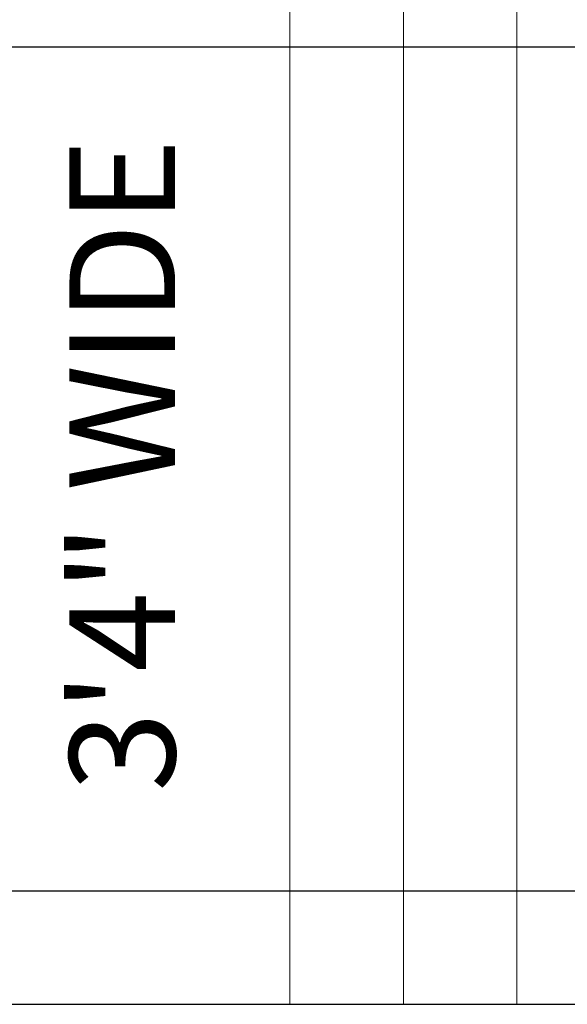
# Model space of a CAD drawing. Units: feet. Extents: x 1654 to 2985, y 1348 to 2230.
# Tile 13 of 53: x 2027 to 2070, y 1565 to 1643. Entities that reach past the tile are written whole.
import ezdxf

# ---------------------------------------------------------------- set-up
doc = ezdxf.new("R2010")
doc.units = ezdxf.units.FT
for name, color, linetype, lineweight in [('A-ANNO-DIMS', 2, 'Continuous', 18), ('A-AREA-IDEN', 7, 'Continuous', 18), ('A-FLOR', 7, 'Continuous', 25), ('A-FLOR-STRS', 7, 'Continuous', 18)]:
    doc.layers.add(name, color=color, linetype=linetype, lineweight=lineweight)
doc.styles.get("Standard").update_dxf_attribs({"font": 'arial.ttf'})
doc.dimstyles.get("Standard").update_dxf_attribs({"dimtxt": 0.18, "dimasz": 0.18, "dimexe": 0.18, "dimexo": 0.0625, "dimgap": 0.09, "dimtad": 0, "dimtih": 1, "dimtoh": 1, "dimdec": 4, "dimzin": 0, "dimdsep": 46, "dimtxsty": 'Standard', "dimcen": 0.09, "dimadec": 0, "dimazin": 0, "dimtfac": 1, "dimtdec": 4, "dimtofl": 0, "dimtmove": 0, "dimatfit": 3, "dimfxl": 1, "dimtolj": 1, "dimtzin": 0, "dimarcsym": 0})

# ---------------------------------------------------------------- blocks, each defined once
blk = doc.blocks.new('*D90')
at = {"layer": 'A-ANNO-DIMS', "color": 0, "lineweight": -2, "transparency": 16777216}
for p, q in [((1852.155, 1641.187), (2242.272, 1641.187)), ((2242.092, 1641.007), (2242.092, 1607.903)), ((2242.092, 1574.435), (2242.092, 1607.539)), ((1852.155, 1574.255), (2242.272, 1574.255))]:
    blk.add_line(p, q, dxfattribs=at)
at = {"layer": 'A-ANNO-DIMS', "color": 0, "transparency": 16777216}
for points in [[(2242.062, 1641.007), (2242.122, 1641.007), (2242.092, 1641.187)], [(2242.062, 1574.435), (2242.122, 1574.435), (2242.092, 1574.255)]]:
    blk.add_solid(points, dxfattribs=at)
at = {"layer": 'Defpoints', "color": 0, "transparency": 16777216}
for p in [(1852.092, 1641.187), (2242.092, 1641.187), (1852.092, 1574.255)]:
    blk.add_point(p, dxfattribs=at)
at = {"layer": 'A-ANNO-DIMS', "color": 0, "transparency": 16777216, "insert": (2242.092, 1607.721), "char_height": 0.18, "attachment_point": 5}
blk.add_mtext('\\A1;66.93', dxfattribs=at)

msp = doc.modelspace()

# ---------------------------------------------------------------- linework, layer by layer
at = {"layer": 'A-FLOR'}
msp.add_line((2008.0924, 1565.2549), (2211.0924, 1565.2549), dxfattribs=at)
at = {"layer": 'A-FLOR-STRS'}
for p, q in [((2048.0924, 1565.2549), (2048.0924, 1661.2549)), ((2057.0924, 1565.2549), (2057.0924, 1661.2549)), ((2066.0924, 1565.2549), (2066.0924, 1661.2549))]:
    msp.add_line(p, q, dxfattribs=at)

# ---------------------------------------------------------------- texts
at = {"layer": 'A-AREA-IDEN'}
msp.add_text('3\'4" WIDE', height=8.38114, rotation=90, dxfattribs=at).set_placement((2038.9942, 1582.1049))

# ---------------------------------------------------------------- dimensions: what is measured, and where the dimension line sits
at = {"layer": 'A-ANNO-DIMS'}
dim = msp.add_linear_dim(base=(2242.0924, 1641.187), p1=(1852.0924, 1574.2549), p2=(1852.0924, 1641.187), angle=90, dimstyle='Standard', override={"dimdec": 2, "dimlfac": 1, "dimrnd": 0, "dimzin": 0, "dimdsep": 46, "dimlunit": 2}, dxfattribs=at)
dim.commit()
dim.dimension.update_dxf_attribs({"geometry": '*D90', "text_midpoint": (2242.0924, 1607.721)})

doc.saveas('drawing.dxf')
